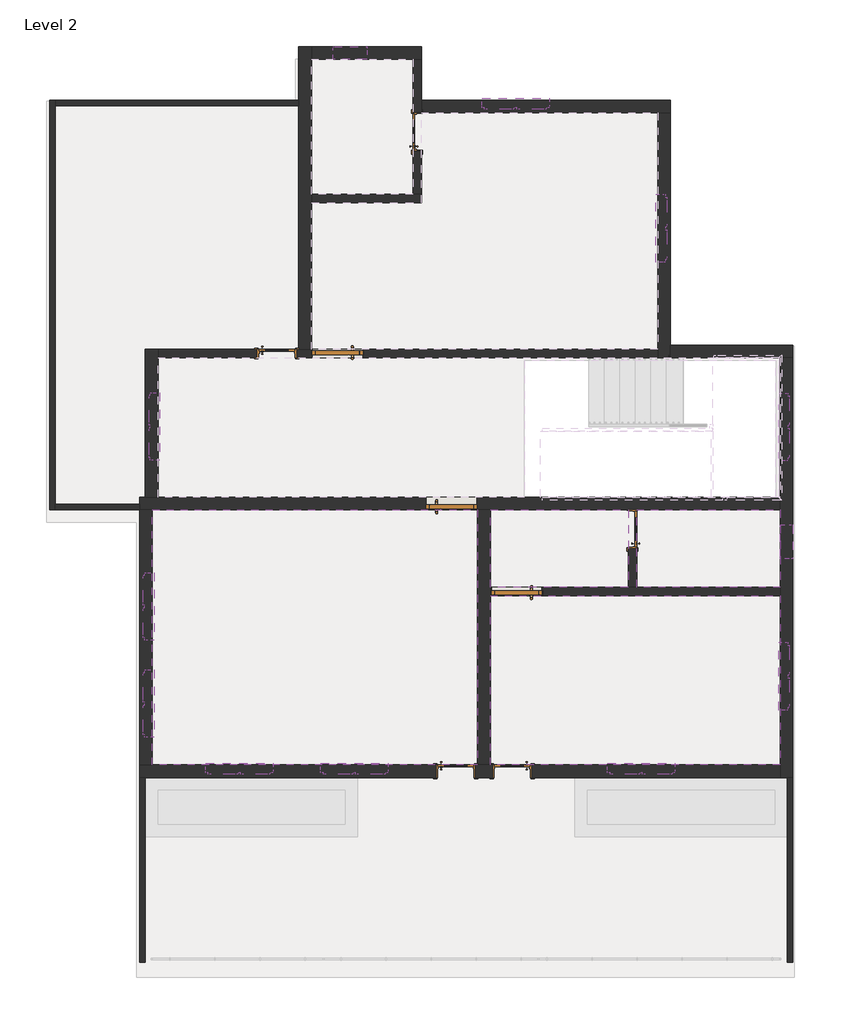
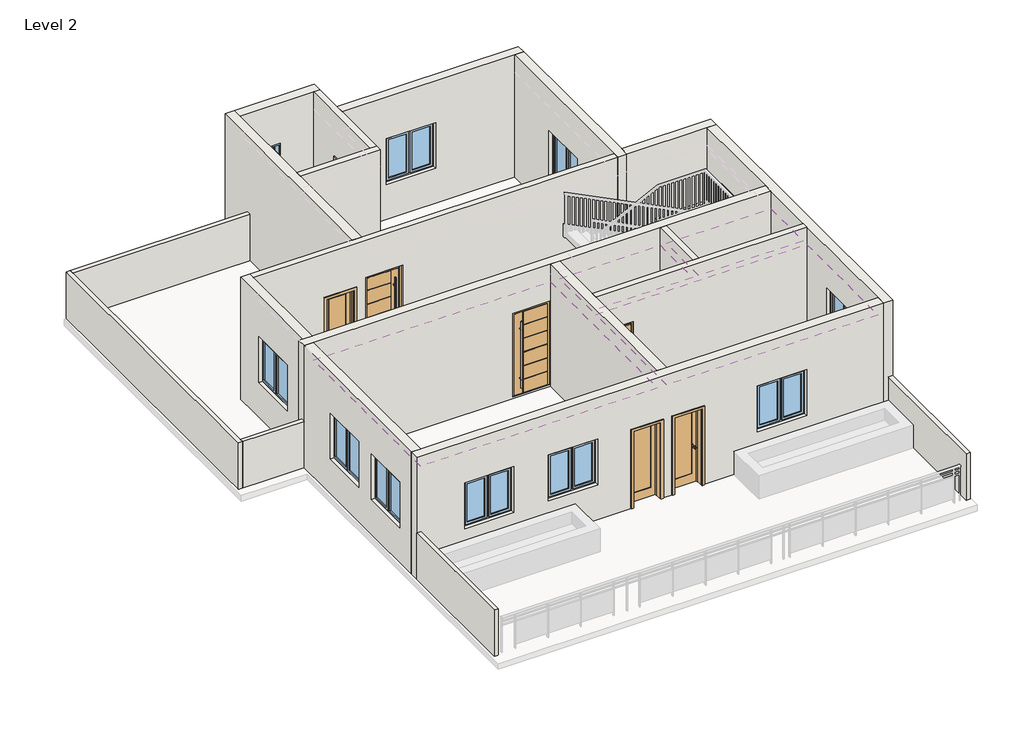
# One storey, part 1 of 3: 21 walls, 12 windows, 8 doors, 4 coverings.
"""IFC4 building model written with IfcOpenShell, lengths in millimetres."""

from ifc_helpers import new_model, si_unit, frame, origin, place, context, project, spatial, polyline, outline, extrude, faceted_brep, transform, mapped, element, save
from components import door_3_5c4206ef, door_3_79df91aa, door_3_130b8d4e, door_69f71937, door_acb0f330, door_a93bef0d, door_ae2d502c, awning_casement_double_4_37d249be, fixed_2_8c8825d0

model = new_model("IFC4")

# Units and contexts
model_context = context("Model", 3, world=origin())
ifc_project = project(units=[si_unit("LENGTHUNIT", "METRE", prefix="MILLI")], contexts=[model_context])

# Site, building, storey
site = spatial("IfcSite", under=ifc_project)
building = spatial("IfcBuilding", under=site)
storey = spatial("IfcBuildingStorey", under=building, Name="Level 2", Elevation=3200.4)

# Coverings
placement = place(None, origin())
element("IfcCovering", 1, ObjectType="2' x 4' ACT System", at=placement, inside=storey, context=model_context, shape_type="SweptSolid", body=[
    extrude(outline(polyline([(-14175.8183666, 640.5503619), (-14175.8183666, -3956.8496381), (-20043.2183666, -3956.8496381), (-20043.2183666, 640.5503619), (-14175.8183666, 640.5503619)])), frame((0.0, 0.0, 6248.4), z_axis=(0.0, 0.0, 1.0), x_axis=(1.0, 0.0, 0.0)), (0.0, 0.0, 1.0), 57.15),
])
element("IfcCovering", 2, ObjectType="2' x 4' ACT System", at=placement, inside=storey, context=model_context, shape_type="SweptSolid", body=[
    extrude(outline(polyline([(-13947.2183666, 640.5503619), (-11458.0183666, 640.5503619), (-11458.0183666, -756.4496381), (-13947.2183666, -756.4496381), (-13947.2183666, 640.5503619)])), frame((0.0, 0.0, 6248.4), z_axis=(0.0, 0.0, 1.0), x_axis=(1.0, 0.0, 0.0)), (0.0, 0.0, 1.0), 57.15),
])
element("IfcCovering", 3, ObjectType="2' x 4' ACT System", at=placement, inside=storey, context=model_context, shape_type="SweptSolid", body=[
    extrude(outline(polyline([(-8714.8183666, 640.5503619), (-8714.8183666, -756.4496381), (-11305.6183666, -756.4496381), (-11305.6183666, 640.5503619), (-8714.8183666, 640.5503619)])), frame((0.0, 0.0, 6248.4), z_axis=(0.0, 0.0, 1.0), x_axis=(1.0, 0.0, 0.0)), (0.0, 0.0, 1.0), 57.15),
])
element("IfcCovering", 4, ObjectType="2' x 4' ACT System", at=placement, inside=storey, context=model_context, shape_type="SweptSolid", body=[
    extrude(outline(polyline([(-13947.2183666, -908.8496381), (-8714.8183666, -908.8496381), (-8714.8183666, -3956.8496381), (-13947.2183666, -3956.8496381), (-13947.2183666, -908.8496381)])), frame((0.0, 0.0, 6248.4), z_axis=(0.0, 0.0, 1.0), x_axis=(1.0, 0.0, 0.0)), (0.0, 0.0, 1.0), 57.15),
])

# Doors
door_3_shape = door_3_5c4206ef(model_context)
element("IfcDoor", 5, ObjectType="3'", at=placement, inside=storey, context=model_context, shape_type="MappedRepresentation", body=[
    mapped(door_3_shape, transform((-13470.9683666, -832.6496381, 3551.4445349), x_axis=(-1.0, 0.0, 0.0), y_axis=(0.0, -1.0, 0.0), z_axis=(0.0, 0.0, 1.0))),
])
door_3_2_shape = door_3_79df91aa(model_context)
element("IfcDoor", 6, ObjectType="3'", at=placement, inside=storey, context=model_context, shape_type="MappedRepresentation", body=[
    mapped(door_3_2_shape, transform((-16703.1183666, 3459.9503619, 3551.4445349), x_axis=(-1.0, 0.0, 0.0), y_axis=(0.0, -1.0, 0.0), z_axis=(0.0, 0.0, 1.0))),
])
door_3_3_shape = door_3_130b8d4e(model_context)
element("IfcDoor", 7, ObjectType="3'", at=placement, inside=storey, context=model_context, shape_type="MappedRepresentation", body=[
    mapped(door_3_3_shape, transform((-14645.7183666, 754.8503619, 3551.4445349), x_axis=(1.0, 0.0, 0.0), y_axis=(0.0, 1.0, 0.0), z_axis=(0.0, 0.0, 1.0))),
])
door_shape = door_69f71937(model_context)
element("IfcDoor", 8, ObjectType="M_Door-Interior-Single-1_Panel-Wood : 2'2\"", at=placement, inside=storey, context=model_context, shape_type="MappedRepresentation", body=[
    mapped(door_shape, transform((-17795.3183666, 3463.1253619, 3505.2), x_axis=(1.0, 0.0, 0.0), y_axis=(0.0, 1.0, 0.0), z_axis=(0.0, 0.0, 1.0))),
])
element("IfcDoor", 9, ObjectType="M_Door-Interior-Single-1_Panel-Wood : 2'2\"", at=placement, inside=storey, context=model_context, shape_type="MappedRepresentation", body=[
    mapped(door_shape, transform((-15271.1933666, 7460.4503619, 3505.2), x_axis=(0.0, 1.0, 0.0), y_axis=(-1.0, 0.0, 0.0), z_axis=(0.0, 0.0, 1.0))),
])
door_2_shape = door_acb0f330(model_context)
element("IfcDoor", 10, ObjectType="M_Door-Interior-Single-1_Panel-Wood : 2'2\"", at=placement, inside=storey, context=model_context, shape_type="MappedRepresentation", body=[
    mapped(door_2_shape, transform((-11378.6433666, 297.6503619, 3505.2), x_axis=(0.0, 1.0, 0.0), y_axis=(-1.0, 0.0, 0.0), z_axis=(0.0, 0.0, 1.0))),
])
door_4_shape = door_a93bef0d(model_context)
element("IfcDoor", 11, ObjectType="M_Door-Interior-Single-1_Panel-Wood : 2'2\"", at=placement, inside=storey, context=model_context, shape_type="MappedRepresentation", body=[
    mapped(door_4_shape, transform((-13553.5183666, -4067.9746381, 3505.2), x_axis=(-1.0, 0.0, 0.0), y_axis=(0.0, -1.0, 0.0), z_axis=(0.0, 0.0, 1.0))),
])
door_5_shape = door_ae2d502c(model_context)
element("IfcDoor", 12, ObjectType="M_Door-Interior-Single-1_Panel-Wood : 2'2\"", at=placement, inside=storey, context=model_context, shape_type="MappedRepresentation", body=[
    mapped(door_5_shape, transform((-14569.5183666, -4067.9746381, 3505.2), x_axis=(1.0, 0.0, 0.0), y_axis=(0.0, 1.0, 0.0), z_axis=(0.0, 0.0, 1.0))),
])

# Walls
element("IfcWall", 13, ObjectType="Generic - 4\"", at=placement, inside=storey, context=model_context, shape_type="Brep", body=[
    faceted_brep([(-21897.4183666, 8031.9503619, 3505.2), (-21897.4183666, 640.5503619, 3505.2), (-21897.4183666, 640.5503619, 4724.4), (-21897.4183666, 8031.9503619, 4724.4), (-21795.8183666, 8031.9503619, 3505.2), (-21795.8183666, 8031.9503619, 4724.4), (-21795.8183666, 7930.3503619, 4724.4), (-21795.8183666, 742.1503619, 4724.4), (-21795.8183666, 640.5503619, 4724.4), (-21795.8183666, 640.5503619, 3505.2), (-21795.8183666, 742.1503619, 3505.2), (-21795.8183666, 7930.3503619, 3505.2)], [[[0, 1, 2, 3]], [[4, 5, 6, 7, 8, 9, 10, 11]], [[1, 0, 4, 11, 10, 9]], [[3, 2, 8, 7, 6, 5]], [[2, 1, 9, 8]], [[0, 3, 5, 4]]]),
])
element("IfcWall", 14, ObjectType="Generic - 4\"", at=placement, inside=storey, context=model_context, shape_type="SweptSolid", body=[
    extrude(outline(polyline([(-20271.8183666, 640.5503619), (-21795.8183666, 640.5503619), (-21795.8183666, 742.1503619), (-20271.8183666, 742.1503619), (-20271.8183666, 640.5503619)])), frame((0.0, 0.0, 3505.2), z_axis=(0.0, 0.0, 1.0), x_axis=(1.0, 0.0, 0.0)), (0.0, 0.0, 1.0), 1219.2),
])
element("IfcWall", 15, ObjectType="Generic - 4\"", at=placement, inside=storey, context=model_context, shape_type="SweptSolid", body=[
    extrude(outline(polyline([(-17401.6183666, 7930.3503619), (-21795.8183666, 7930.3503619), (-21795.8183666, 8031.9503619), (-17401.6183666, 8031.9503619), (-17401.6183666, 7930.3503619)])), frame((0.0, 0.0, 3505.2), z_axis=(0.0, 0.0, 1.0), x_axis=(1.0, 0.0, 0.0)), (0.0, 0.0, 1.0), 1219.2),
])
element("IfcWall", 16, ObjectType="Generic - 4\"", at=placement, inside=storey, context=model_context, shape_type="SweptSolid", body=[
    extrude(outline(polyline([(-20271.8183666, -7512.8496381), (-20271.8183666, -4185.4496381), (-20170.2183666, -4185.4496381), (-20170.2183666, -7512.8496381), (-20271.8183666, -7512.8496381)])), frame((0.0, 0.0, 3505.2), z_axis=(0.0, 0.0, 1.0), x_axis=(1.0, 0.0, 0.0)), (0.0, 0.0, 1.0), 1219.2),
])
element("IfcWall", 17, ObjectType="Generic - 4\"", at=placement, inside=storey, context=model_context, shape_type="SweptSolid", body=[
    extrude(outline(polyline([(-8486.2183666, -4185.4496381), (-8486.2183666, -7512.8496381), (-8587.8183666, -7512.8496381), (-8587.8183666, -4185.4496381), (-8486.2183666, -4185.4496381)])), frame((0.0, 0.0, 3505.2), z_axis=(0.0, 0.0, 1.0), x_axis=(1.0, 0.0, 0.0)), (0.0, 0.0, 1.0), 1219.2),
])
element("IfcWall", 18, ObjectType="Generic - 6\"", at=placement, inside=storey, context=model_context, shape_type="Brep", body=[
    faceted_brep([(-15344.2183666, 6330.1503619, 6705.6), (-15344.2183666, 8768.5503619, 6705.6), (-15344.2183666, 8768.5503619, 3505.2), (-15344.2183666, 7815.6503619, 3505.2), (-15344.2183666, 7815.6503619, 5530.2), (-15344.2183666, 7105.2503619, 5530.2), (-15344.2183666, 7105.2503619, 3505.2), (-15344.2183666, 6330.1503619, 3505.2), (-15191.8183666, 8768.5503619, 6705.6), (-15191.8183666, 8031.9503619, 6705.6), (-15191.8183666, 7803.3503619, 6705.6), (-15191.8183666, 6330.1503619, 6705.6), (-15191.8183666, 6330.1503619, 3505.2), (-15191.8183666, 7105.2503619, 3505.2), (-15191.8183666, 7105.2503619, 5530.2), (-15191.8183666, 7815.6503619, 5530.2), (-15191.8183666, 7815.6503619, 3505.2), (-15191.8183666, 8031.9503619, 3505.2), (-15191.8183666, 8768.5503619, 3505.2)], [[[0, 1, 2, 3, 4, 5, 6, 7]], [[8, 9, 10, 11, 12, 13, 14, 15, 16, 17, 18]], [[2, 18, 17, 16, 3]], [[12, 7, 6, 13]], [[1, 0, 11, 10, 9, 8]], [[2, 1, 8, 18]], [[0, 7, 12, 11]], [[15, 4, 3, 16]], [[4, 15, 14, 5]], [[5, 14, 13, 6]]]),
])
element("IfcWall", 19, ObjectType="Generic - 6\"", at=placement, inside=storey, context=model_context, shape_type="Brep", body=[
    faceted_brep([(-10924.6183666, 3383.7503619, 6705.6), (-19941.6183666, 3383.7503619, 6705.6), (-19941.6183666, 3383.7503619, 3505.2), (-18150.5183666, 3383.7503619, 3505.2), (-18150.5183666, 3383.7503619, 5530.2), (-17440.1183666, 3383.7503619, 5530.2), (-17440.1183666, 3383.7503619, 3505.2), (-10924.6183666, 3383.7503619, 3505.2), (-17160.3183666, 3383.7503619, 5740.9445349), (-16245.9183666, 3383.7503619, 5740.9445349), (-16245.9183666, 3383.7503619, 3551.4445349), (-17160.3183666, 3383.7503619, 3551.4445349), (-19941.6183666, 3536.1503619, 6705.6), (-17401.6183666, 3536.1503619, 6705.6), (-17173.0183666, 3536.1503619, 6705.6), (-10924.6183666, 3536.1503619, 6705.6), (-10924.6183666, 3536.1503619, 3505.2), (-17173.0183666, 3536.1503619, 3505.2), (-17401.6183666, 3536.1503619, 3505.2), (-17440.1183666, 3536.1503619, 3505.2), (-17440.1183666, 3536.1503619, 5530.2), (-18150.5183666, 3536.1503619, 5530.2), (-18150.5183666, 3536.1503619, 3505.2), (-19941.6183666, 3536.1503619, 3505.2), (-16245.9183666, 3536.1503619, 5740.9445349), (-17160.3183666, 3536.1503619, 5740.9445349), (-17160.3183666, 3536.1503619, 3551.4445349), (-16245.9183666, 3536.1503619, 3551.4445349), (-16245.9183666, 3516.1503619, 5740.9445349), (-17160.3183666, 3516.1503619, 5740.9445349), (-17160.3183666, 3439.1503619, 5740.9445349), (-16245.9183666, 3439.1503619, 5740.9445349), (-17160.3183666, 3516.1503619, 3551.4445349), (-17160.3183666, 3439.1503619, 3551.4445349), (-17175.3183666, 3516.1503619, 3551.4445349), (-17175.3183666, 3439.1503619, 3551.4445349), (-16245.9183666, 3439.1503619, 3551.4445349), (-16230.9183666, 3439.1503619, 3551.4445349), (-16230.9183666, 3516.1503619, 3551.4445349), (-16245.9183666, 3516.1503619, 3551.4445349), (-16230.9183666, 3516.1503619, 5755.9445349), (-16230.9183666, 3439.1503619, 5755.9445349), (-17175.3183666, 3439.1503619, 5755.9445349), (-17175.3183666, 3516.1503619, 5755.9445349)], [[[0, 1, 2, 3, 4, 5, 6, 7], [8, 9, 10, 11]], [[12, 13, 14, 15, 16, 17, 18, 19, 20, 21, 22, 23], [24, 25, 26, 27]], [[2, 23, 22, 3]], [[16, 7, 6, 19, 18, 17]], [[1, 0, 15, 14, 13, 12]], [[0, 7, 16, 15]], [[2, 1, 12, 23]], [[5, 20, 19, 6]], [[20, 5, 4, 21]], [[21, 4, 3, 22]], [[24, 28, 29, 25]], [[8, 30, 31, 9]], [[25, 29, 32, 26]], [[30, 8, 11, 33]], [[26, 32, 34, 35, 33, 11, 10, 36, 37, 38, 39, 27]], [[28, 24, 27, 39]], [[9, 31, 36, 10]], [[40, 41, 42, 43]], [[35, 34, 43, 42]], [[31, 30, 33, 35, 42, 41, 37, 36]], [[38, 37, 41, 40]], [[29, 28, 39, 38, 40, 43, 34, 32]]]),
])
element("IfcWall", 20, ObjectType="Generic - 6\"", at=placement, inside=storey, context=model_context, shape_type="Brep", body=[
    faceted_brep([(-17173.0183666, 6177.7503619, 3505.2), (-15191.8183666, 6177.7503619, 3505.2), (-15191.8183666, 6177.7503619, 6705.6), (-17173.0183666, 6177.7503619, 6705.6), (-17173.0183666, 6330.1503619, 3505.2), (-17173.0183666, 6330.1503619, 6705.6), (-15344.2183666, 6330.1503619, 6705.6), (-15191.8183666, 6330.1503619, 6705.6), (-15191.8183666, 6330.1503619, 3505.2), (-15344.2183666, 6330.1503619, 3505.2)], [[[0, 1, 2, 3]], [[4, 5, 6, 7, 8, 9]], [[1, 0, 4, 9, 8]], [[3, 2, 7, 6, 5]], [[0, 3, 5, 4]], [[2, 1, 8, 7]]]),
])
element("IfcWall", 21, ObjectType="Generic - 6\"", at=placement, inside=storey, context=model_context, shape_type="Brep", body=[
    faceted_brep([(-8714.8183666, -756.4496381, 3505.2), (-11305.6183666, -756.4496381, 3505.2), (-11458.0183666, -756.4496381, 3505.2), (-13947.2183666, -756.4496381, 3505.2), (-13947.2183666, -756.4496381, 6705.6), (-11458.0183666, -756.4496381, 6705.6), (-11305.6183666, -756.4496381, 6705.6), (-8714.8183666, -756.4496381, 6705.6), (-13013.7683666, -756.4496381, 5740.9445349), (-13928.1683666, -756.4496381, 5740.9445349), (-13928.1683666, -756.4496381, 3551.4445349), (-13013.7683666, -756.4496381, 3551.4445349), (-13947.2183666, -908.8496381, 3505.2), (-8714.8183666, -908.8496381, 3505.2), (-8714.8183666, -908.8496381, 6705.6), (-13947.2183666, -908.8496381, 6705.6), (-13928.1683666, -908.8496381, 5740.9445349), (-13013.7683666, -908.8496381, 5740.9445349), (-13013.7683666, -908.8496381, 3551.4445349), (-13928.1683666, -908.8496381, 3551.4445349), (-13928.1683666, -888.8496381, 5740.9445349), (-13013.7683666, -888.8496381, 5740.9445349), (-13013.7683666, -811.8496381, 5740.9445349), (-13928.1683666, -811.8496381, 5740.9445349), (-13928.1683666, -888.8496381, 3551.4445349), (-13928.1683666, -811.8496381, 3551.4445349), (-13013.7683666, -888.8496381, 3551.4445349), (-12998.7683666, -888.8496381, 3551.4445349), (-12998.7683666, -811.8496381, 3551.4445349), (-13013.7683666, -811.8496381, 3551.4445349), (-13943.1683666, -811.8496381, 3551.4445349), (-13943.1683666, -888.8496381, 3551.4445349), (-12998.7683666, -888.8496381, 5755.9445349), (-13943.1683666, -888.8496381, 5755.9445349), (-13943.1683666, -811.8496381, 5755.9445349), (-12998.7683666, -811.8496381, 5755.9445349)], [[[0, 1, 2, 3, 4, 5, 6, 7], [8, 9, 10, 11]], [[12, 13, 14, 15], [16, 17, 18, 19]], [[3, 2, 1, 0, 13, 12]], [[7, 6, 5, 4, 15, 14]], [[0, 7, 14, 13]], [[4, 3, 12, 15]], [[16, 20, 21, 17]], [[8, 22, 23, 9]], [[20, 16, 19, 24]], [[9, 23, 25, 10]], [[24, 19, 18, 26, 27, 28, 29, 11, 10, 25, 30, 31]], [[17, 21, 26, 18]], [[22, 8, 11, 29]], [[32, 33, 34, 35]], [[31, 30, 34, 33]], [[23, 22, 29, 28, 35, 34, 30, 25]], [[28, 27, 32, 35]], [[21, 20, 24, 31, 33, 32, 27, 26]]]),
])
element("IfcWall", 22, ObjectType="Generic - 6\"", at=placement, inside=storey, context=model_context, shape_type="SweptSolid", body=[
    extrude(outline(polyline([(-756.4496381, 6705.6), (640.5503619, 6705.6), (640.5503619, 5530.2), (-57.5496381, 5530.2), (-57.5496381, 3505.2), (-756.4496381, 3505.2), (-756.4496381, 6705.6)])), frame((-11458.0183666, 0.0, 0.0), z_axis=(1.0, 0.0, 0.0), x_axis=(0.0, 1.0, 0.0)), (0.0, 0.0, 1.0), 152.4),
])
element("IfcWall", 23, ObjectType="Generic - 9\"", at=placement, inside=storey, context=model_context, shape_type="Brep", body=[
    faceted_brep([(-17173.0183666, 3536.1503619, 3505.2), (-17173.0183666, 6177.7503619, 3505.2), (-17173.0183666, 6330.1503619, 3505.2), (-17173.0183666, 8768.5503619, 3505.2), (-17173.0183666, 8997.1503619, 3505.2), (-17173.0183666, 8997.1503619, 6705.6), (-17173.0183666, 8768.5503619, 6705.6), (-17173.0183666, 6330.1503619, 6705.6), (-17173.0183666, 6177.7503619, 6705.6), (-17173.0183666, 3536.1503619, 6705.6), (-17401.6183666, 3536.1503619, 3505.2), (-17401.6183666, 3536.1503619, 6705.6), (-17401.6183666, 8997.1503619, 6705.6), (-17401.6183666, 8997.1503619, 3505.2), (-17401.6183666, 8031.9503619, 3505.2), (-17401.6183666, 7930.3503619, 3505.2)], [[[0, 1, 2, 3, 4, 5, 6, 7, 8, 9]], [[10, 11, 12, 13, 14, 15]], [[4, 3, 2, 1, 0, 10, 15, 14, 13]], [[9, 8, 7, 6, 5, 12, 11]], [[5, 4, 13, 12]], [[0, 9, 11, 10]]]),
])
element("IfcWall", 24, ObjectType="Generic - 9\"", at=placement, inside=storey, context=model_context, shape_type="Brep", body=[
    faceted_brep([(-17173.0183666, 8768.5503619, 3505.2), (-15344.2183666, 8768.5503619, 3505.2), (-15191.8183666, 8768.5503619, 3505.2), (-15191.8183666, 8768.5503619, 6705.6), (-15344.2183666, 8768.5503619, 6705.6), (-17173.0183666, 8768.5503619, 6705.6), (-16169.7183666, 8768.5503619, 5638.8), (-16169.7183666, 8768.5503619, 5334.0), (-16779.3183666, 8768.5503619, 5334.0), (-16779.3183666, 8768.5503619, 5638.8), (-17173.0183666, 8997.1503619, 3505.2), (-17173.0183666, 8997.1503619, 6705.6), (-15191.8183666, 8997.1503619, 6705.6), (-15191.8183666, 8997.1503619, 3505.2), (-16169.7183666, 8997.1503619, 5638.8), (-16779.3183666, 8997.1503619, 5638.8), (-16779.3183666, 8997.1503619, 5334.0), (-16169.7183666, 8997.1503619, 5334.0)], [[[0, 1, 2, 3, 4, 5], [6, 7, 8, 9]], [[10, 11, 12, 13], [14, 15, 16, 17]], [[2, 1, 0, 10, 13]], [[5, 4, 3, 12, 11]], [[0, 5, 11, 10]], [[3, 2, 13, 12]], [[7, 6, 14, 17]], [[8, 7, 17, 16]], [[9, 8, 16, 15]], [[6, 9, 15, 14]]]),
])
element("IfcWall", 25, ObjectType="Generic - 9\"", at=placement, inside=storey, context=model_context, shape_type="Brep", body=[
    faceted_brep([(-15191.8183666, 7803.3503619, 3505.2), (-10924.6183666, 7803.3503619, 3505.2), (-10696.0183666, 7803.3503619, 3505.2), (-10696.0183666, 7803.3503619, 6705.6), (-10924.6183666, 7803.3503619, 6705.6), (-15191.8183666, 7803.3503619, 6705.6), (-14099.6183666, 7803.3503619, 4419.6), (-14099.6183666, 7803.3503619, 5619.6), (-12880.4183666, 7803.3503619, 5619.6), (-12880.4183666, 7803.3503619, 4419.6), (-15191.8183666, 8031.9503619, 3505.2), (-15191.8183666, 8031.9503619, 6705.6), (-10696.0183666, 8031.9503619, 6705.6), (-10696.0183666, 8031.9503619, 3505.2), (-14099.6183666, 8031.9503619, 4419.6), (-12880.4183666, 8031.9503619, 4419.6), (-12880.4183666, 8031.9503619, 5619.6), (-14099.6183666, 8031.9503619, 5619.6)], [[[0, 1, 2, 3, 4, 5], [6, 7, 8, 9]], [[10, 11, 12, 13], [14, 15, 16, 17]], [[2, 1, 0, 10, 13]], [[5, 4, 3, 12, 11]], [[0, 5, 11, 10]], [[3, 2, 13, 12]], [[7, 6, 14, 17]], [[8, 7, 17, 16]], [[9, 8, 16, 15]], [[6, 9, 15, 14]]]),
])
element("IfcWall", 26, ObjectType="Generic - 9\"", at=placement, inside=storey, context=model_context, shape_type="Brep", body=[
    faceted_brep([(-10924.6183666, 7803.3503619, 3505.2), (-10924.6183666, 3536.1503619, 3505.2), (-10924.6183666, 3383.7503619, 3505.2), (-10924.6183666, 3383.7503619, 6705.6), (-10924.6183666, 3536.1503619, 6705.6), (-10924.6183666, 7803.3503619, 6705.6), (-10924.6183666, 5110.9503619, 4419.6), (-10924.6183666, 6330.1503619, 4419.6), (-10924.6183666, 6330.1503619, 5619.6), (-10924.6183666, 5110.9503619, 5619.6), (-10696.0183666, 7803.3503619, 3505.2), (-10696.0183666, 7803.3503619, 6705.6), (-10696.0183666, 3612.3503619, 6705.6), (-10696.0183666, 3383.7503619, 6705.6), (-10696.0183666, 3383.7503619, 3505.2), (-10696.0183666, 3612.3503619, 3505.2), (-10696.0183666, 5110.9503619, 4419.6), (-10696.0183666, 5110.9503619, 5619.6), (-10696.0183666, 6330.1503619, 5619.6), (-10696.0183666, 6330.1503619, 4419.6)], [[[0, 1, 2, 3, 4, 5], [6, 7, 8, 9]], [[10, 11, 12, 13, 14, 15], [16, 17, 18, 19]], [[2, 1, 0, 10, 15, 14]], [[5, 4, 3, 13, 12, 11]], [[0, 5, 11, 10]], [[3, 2, 14, 13]], [[17, 16, 6, 9]], [[18, 17, 9, 8]], [[19, 18, 8, 7]], [[16, 19, 7, 6]]]),
])
element("IfcWall", 27, ObjectType="Generic - 9\"", at=placement, inside=storey, context=model_context, shape_type="Brep", body=[
    faceted_brep([(-10696.0183666, 3383.7503619, 3505.2), (-8714.8183666, 3383.7503619, 3505.2), (-8486.2183666, 3383.7503619, 3505.2), (-8486.2183666, 3383.7503619, 6705.6), (-8714.8183666, 3383.7503619, 6705.6), (-10696.0183666, 3383.7503619, 6705.6), (-10696.0183666, 3612.3503619, 3505.2), (-10696.0183666, 3612.3503619, 6705.6), (-8486.2183666, 3612.3503619, 6705.6), (-8486.2183666, 3612.3503619, 3505.2)], [[[0, 1, 2, 3, 4, 5]], [[6, 7, 8, 9]], [[2, 1, 0, 6, 9]], [[5, 4, 3, 8, 7]], [[0, 5, 7, 6]], [[3, 2, 9, 8]]]),
])
element("IfcWall", 28, ObjectType="Generic - 9\"", at=placement, inside=storey, context=model_context, shape_type="Brep", body=[
    faceted_brep([(-8714.8183666, 3383.7503619, 3505.2), (-8714.8183666, 869.1503619, 3505.2), (-8714.8183666, 640.5503619, 3505.2), (-8714.8183666, -756.4496381, 3505.2), (-8714.8183666, -908.8496381, 3505.2), (-8714.8183666, -3956.8496381, 3505.2), (-8714.8183666, -4185.4496381, 3505.2), (-8714.8183666, -4185.4496381, 6705.6), (-8714.8183666, -3956.8496381, 6705.6), (-8714.8183666, -908.8496381, 6705.6), (-8714.8183666, -756.4496381, 6705.6), (-8714.8183666, 640.5503619, 6705.6), (-8714.8183666, 869.1503619, 6705.6), (-8714.8183666, 3383.7503619, 6705.6), (-8714.8183666, -2966.2496381, 4419.6), (-8714.8183666, -1747.0496381, 4419.6), (-8714.8183666, -1747.0496381, 5619.6), (-8714.8183666, -2966.2496381, 5619.6), (-8714.8183666, 1529.5503619, 4419.6), (-8714.8183666, 2748.7503619, 4419.6), (-8714.8183666, 2748.7503619, 5619.6), (-8714.8183666, 1529.5503619, 5619.6), (-8714.8183666, -235.7496381, 5638.8), (-8714.8183666, -235.7496381, 5334.0), (-8714.8183666, 373.8503619, 5334.0), (-8714.8183666, 373.8503619, 5638.8), (-8486.2183666, 3383.7503619, 3505.2), (-8486.2183666, 3383.7503619, 6705.6), (-8486.2183666, -4185.4496381, 6705.6), (-8486.2183666, -4185.4496381, 4724.4), (-8486.2183666, -4185.4496381, 3505.2), (-8486.2183666, -2966.2496381, 4419.6), (-8486.2183666, -2966.2496381, 5619.6), (-8486.2183666, -1747.0496381, 5619.6), (-8486.2183666, -1747.0496381, 4419.6), (-8486.2183666, 1529.5503619, 4419.6), (-8486.2183666, 1529.5503619, 5619.6), (-8486.2183666, 2748.7503619, 5619.6), (-8486.2183666, 2748.7503619, 4419.6), (-8486.2183666, -235.7496381, 5638.8), (-8486.2183666, 373.8503619, 5638.8), (-8486.2183666, 373.8503619, 5334.0), (-8486.2183666, -235.7496381, 5334.0), (-8587.8183666, -4185.4496381, 3505.2)], [[[0, 1, 2, 3, 4, 5, 6, 7, 8, 9, 10, 11, 12, 13], [14, 15, 16, 17], [18, 19, 20, 21], [22, 23, 24, 25]], [[26, 27, 28, 29, 30], [31, 32, 33, 34], [35, 36, 37, 38], [39, 40, 41, 42]], [[6, 5, 4, 3, 2, 1, 0, 26, 30, 43]], [[13, 12, 11, 10, 9, 8, 7, 28, 27]], [[0, 13, 27, 26]], [[6, 43, 30, 29, 28, 7]], [[32, 31, 14, 17]], [[33, 32, 17, 16]], [[34, 33, 16, 15]], [[31, 34, 15, 14]], [[36, 35, 18, 21]], [[37, 36, 21, 20]], [[38, 37, 20, 19]], [[35, 38, 19, 18]], [[23, 22, 39, 42]], [[24, 23, 42, 41]], [[25, 24, 41, 40]], [[22, 25, 40, 39]]]),
])
element("IfcWall", 29, ObjectType="Generic - 9\"", at=placement, inside=storey, context=model_context, shape_type="Brep", body=[
    faceted_brep([(-20272.0228179, -3956.8496381, 3505.2), (-20272.0228179, -3956.8496381, 6705.6), (-20271.8183666, -3956.8496381, 6705.6), (-20043.2183666, -3956.8496381, 6705.6), (-14175.8183666, -3956.8496381, 6705.6), (-13947.2183666, -3956.8496381, 6705.6), (-8714.8183666, -3956.8496381, 6705.6), (-8714.8183666, -3956.8496381, 3505.2), (-13198.3183666, -3956.8496381, 3505.2), (-13198.3183666, -3956.8496381, 5530.2), (-13908.7183666, -3956.8496381, 5530.2), (-13908.7183666, -3956.8496381, 3505.2), (-13947.2183666, -3956.8496381, 3505.2), (-14175.8183666, -3956.8496381, 3505.2), (-14214.3183666, -3956.8496381, 3505.2), (-14214.3183666, -3956.8496381, 5530.2), (-14924.7183666, -3956.8496381, 5530.2), (-14924.7183666, -3956.8496381, 3505.2), (-20043.2183666, -3956.8496381, 3505.2), (-20271.8183666, -3956.8496381, 3505.2), (-19084.3683666, -3956.8496381, 4419.6), (-17865.1683666, -3956.8496381, 4419.6), (-17865.1683666, -3956.8496381, 5619.6), (-19084.3683666, -3956.8496381, 5619.6), (-17007.9183666, -3956.8496381, 4419.6), (-15788.7183666, -3956.8496381, 4419.6), (-15788.7183666, -3956.8496381, 5619.6), (-17007.9183666, -3956.8496381, 5619.6), (-11832.6683666, -3956.8496381, 4419.6), (-10613.4683666, -3956.8496381, 4419.6), (-10613.4683666, -3956.8496381, 5619.6), (-11832.6683666, -3956.8496381, 5619.6), (-20272.0228179, -4185.4496381, 6705.6), (-20272.0228179, -4185.4496381, 3505.2), (-20271.8183666, -4185.4496381, 3505.2), (-20170.2183666, -4185.4496381, 3505.2), (-14924.7183666, -4185.4496381, 3505.2), (-14924.7183666, -4185.4496381, 5530.2), (-14214.3183666, -4185.4496381, 5530.2), (-14214.3183666, -4185.4496381, 3505.2), (-13908.7183666, -4185.4496381, 3505.2), (-13908.7183666, -4185.4496381, 5530.2), (-13198.3183666, -4185.4496381, 5530.2), (-13198.3183666, -4185.4496381, 3505.2), (-8714.8183666, -4185.4496381, 3505.2), (-8714.8183666, -4185.4496381, 6705.6), (-19084.3683666, -4185.4496381, 4419.6), (-19084.3683666, -4185.4496381, 5619.6), (-17865.1683666, -4185.4496381, 5619.6), (-17865.1683666, -4185.4496381, 4419.6), (-17007.9183666, -4185.4496381, 4419.6), (-17007.9183666, -4185.4496381, 5619.6), (-15788.7183666, -4185.4496381, 5619.6), (-15788.7183666, -4185.4496381, 4419.6), (-11832.6683666, -4185.4496381, 4419.6), (-11832.6683666, -4185.4496381, 5619.6), (-10613.4683666, -4185.4496381, 5619.6), (-10613.4683666, -4185.4496381, 4419.6)], [[[0, 1, 2, 3, 4, 5, 6, 7, 8, 9, 10, 11, 12, 13, 14, 15, 16, 17, 18, 19], [20, 21, 22, 23], [24, 25, 26, 27], [28, 29, 30, 31]], [[32, 33, 34, 35, 36, 37, 38, 39, 40, 41, 42, 43, 44, 45], [46, 47, 48, 49], [50, 51, 52, 53], [54, 55, 56, 57]], [[33, 0, 19, 18, 17, 36, 35, 34]], [[7, 44, 43, 8]], [[39, 14, 13, 12, 11, 40]], [[1, 0, 33, 32]], [[6, 5, 4, 3, 2, 1, 32, 45]], [[6, 45, 44, 7]], [[47, 46, 20, 23]], [[48, 47, 23, 22]], [[49, 48, 22, 21]], [[46, 49, 21, 20]], [[51, 50, 24, 27]], [[52, 51, 27, 26]], [[53, 52, 26, 25]], [[50, 53, 25, 24]], [[55, 54, 28, 31]], [[56, 55, 31, 30]], [[57, 56, 30, 29]], [[54, 57, 29, 28]], [[15, 14, 39, 38]], [[16, 15, 38, 37]], [[17, 16, 37, 36]], [[10, 41, 40, 11]], [[41, 10, 9, 42]], [[42, 9, 8, 43]]]),
])
element("IfcWall", 30, ObjectType="Generic - 9\"", at=placement, inside=storey, context=model_context, shape_type="SweptSolid", body=[
    extrude(outline(polyline([(-3956.8496381, 3505.2), (-3956.8496381, 6705.6), (640.5503619, 6705.6), (640.5503619, 3505.2), (-3956.8496381, 3505.2)]), holes=[polyline([(-489.7496381, 4419.6), (-489.7496381, 5619.6), (-1708.9496381, 5619.6), (-1708.9496381, 4419.6), (-489.7496381, 4419.6)]), polyline([(-2242.3496381, 4419.6), (-2242.3496381, 5619.6), (-3461.5496381, 5619.6), (-3461.5496381, 4419.6), (-2242.3496381, 4419.6)])]), frame((-20271.8183666, 0.0, 0.0), z_axis=(1.0, 0.0, 0.0), x_axis=(0.0, 1.0, 0.0)), (0.0, 0.0, 1.0), 228.6),
])
element("IfcWall", 31, ObjectType="Generic - 9\"", at=placement, inside=storey, context=model_context, shape_type="Brep", body=[
    faceted_brep([(-8714.8183666, 640.5503619, 6705.6), (-11305.6183666, 640.5503619, 6705.6), (-11458.0183666, 640.5503619, 6705.6), (-13947.2183666, 640.5503619, 6705.6), (-14175.8183666, 640.5503619, 6705.6), (-20043.2183666, 640.5503619, 6705.6), (-20271.8183666, 640.5503619, 6705.6), (-20271.8183666, 640.5503619, 4724.4), (-20271.8183666, 640.5503619, 3505.2), (-20043.2183666, 640.5503619, 3505.2), (-14175.8183666, 640.5503619, 3505.2), (-13947.2183666, 640.5503619, 3505.2), (-11458.0183666, 640.5503619, 3505.2), (-11458.0183666, 640.5503619, 5530.2), (-11305.6183666, 640.5503619, 5530.2), (-11305.6183666, 640.5503619, 3505.2), (-8714.8183666, 640.5503619, 3505.2), (-15102.9183666, 640.5503619, 5740.9445349), (-14188.5183666, 640.5503619, 5740.9445349), (-14188.5183666, 640.5503619, 3551.4445349), (-15102.9183666, 640.5503619, 3551.4445349), (-8714.8183666, 869.1503619, 3505.2), (-19941.6183666, 869.1503619, 3505.2), (-20170.2183666, 869.1503619, 3505.2), (-20271.8183666, 869.1503619, 3505.2), (-20271.8183666, 869.1503619, 6705.6), (-20170.2183666, 869.1503619, 6705.6), (-19941.6183666, 869.1503619, 6705.6), (-8714.8183666, 869.1503619, 6705.6), (-14188.5183666, 869.1503619, 5740.9445349), (-15102.9183666, 869.1503619, 5740.9445349), (-15102.9183666, 869.1503619, 3551.4445349), (-14188.5183666, 869.1503619, 3551.4445349), (-11305.6183666, 652.8503619, 3505.2), (-11458.0183666, 652.8503619, 3505.2), (-20271.8183666, 742.1503619, 3505.2), (-11305.6183666, 652.8503619, 5530.2), (-11458.0183666, 652.8503619, 5530.2), (-15102.9183666, 660.5503619, 5740.9445349), (-14188.5183666, 660.5503619, 5740.9445349), (-14188.5183666, 737.5503619, 5740.9445349), (-15102.9183666, 737.5503619, 5740.9445349), (-14188.5183666, 660.5503619, 3551.4445349), (-14188.5183666, 737.5503619, 3551.4445349), (-14173.5183666, 660.5503619, 3551.4445349), (-14173.5183666, 737.5503619, 3551.4445349), (-15102.9183666, 737.5503619, 3551.4445349), (-15117.9183666, 737.5503619, 3551.4445349), (-15117.9183666, 660.5503619, 3551.4445349), (-15102.9183666, 660.5503619, 3551.4445349), (-15117.9183666, 660.5503619, 5755.9445349), (-15117.9183666, 737.5503619, 5755.9445349), (-14173.5183666, 737.5503619, 5755.9445349), (-14173.5183666, 660.5503619, 5755.9445349)], [[[0, 1, 2, 3, 4, 5, 6, 7, 8, 9, 10, 11, 12, 13, 14, 15, 16], [17, 18, 19, 20]], [[21, 22, 23, 24, 25, 26, 27, 28], [29, 30, 31, 32]], [[24, 23, 22, 21, 16, 15, 33, 34, 12, 11, 10, 9, 8, 35]], [[6, 5, 4, 3, 2, 1, 0, 28, 27, 26, 25]], [[24, 35, 8, 7, 6, 25]], [[0, 16, 21, 28]], [[36, 33, 15, 14]], [[34, 37, 13, 12]], [[37, 36, 14, 13]], [[17, 38, 39, 18]], [[29, 40, 41, 30]], [[18, 39, 42, 19]], [[40, 29, 32, 43]], [[19, 42, 44, 45, 43, 32, 31, 46, 47, 48, 49, 20]], [[38, 17, 20, 49]], [[30, 41, 46, 31]], [[50, 51, 52, 53]], [[45, 44, 53, 52]], [[41, 40, 43, 45, 52, 51, 47, 46]], [[48, 47, 51, 50]], [[39, 38, 49, 48, 50, 53, 44, 42]], [[33, 36, 37, 34]]]),
])
element("IfcWall", 32, ObjectType="Generic - 9\"", at=placement, inside=storey, context=model_context, shape_type="Brep", body=[
    faceted_brep([(-19941.6183666, 869.1503619, 6705.6), (-19941.6183666, 869.1503619, 3505.2), (-19941.6183666, 3383.7503619, 3505.2), (-19941.6183666, 3536.1503619, 3505.2), (-19941.6183666, 3536.1503619, 6705.6), (-19941.6183666, 3383.7503619, 6705.6), (-19941.6183666, 2755.1003619, 4419.6), (-19941.6183666, 1535.9003619, 4419.6), (-19941.6183666, 1535.9003619, 5619.6), (-19941.6183666, 2755.1003619, 5619.6), (-20170.2183666, 869.1503619, 3505.2), (-20170.2183666, 869.1503619, 6705.6), (-20170.2183666, 3536.1503619, 6705.6), (-20170.2183666, 3536.1503619, 3505.2), (-20170.2183666, 2755.1003619, 4419.6), (-20170.2183666, 2755.1003619, 5619.6), (-20170.2183666, 1535.9003619, 5619.6), (-20170.2183666, 1535.9003619, 4419.6)], [[[0, 1, 2, 3, 4, 5], [6, 7, 8, 9]], [[10, 11, 12, 13], [14, 15, 16, 17]], [[3, 2, 1, 10, 13]], [[0, 5, 4, 12, 11]], [[0, 11, 10, 1]], [[4, 3, 13, 12]], [[15, 14, 6, 9]], [[16, 15, 9, 8]], [[17, 16, 8, 7]], [[14, 17, 7, 6]]]),
])
element("IfcWall", 33, ObjectType="Generic - 9\"", at=placement, inside=storey, context=model_context, shape_type="Brep", body=[
    faceted_brep([(-13947.2183666, -3956.8496381, 3505.2), (-13947.2183666, -908.8496381, 3505.2), (-13947.2183666, -756.4496381, 3505.2), (-13947.2183666, 640.5503619, 3505.2), (-13947.2183666, 640.5503619, 6705.6), (-13947.2183666, -756.4496381, 6705.6), (-13947.2183666, -908.8496381, 6705.6), (-13947.2183666, -3956.8496381, 6705.6), (-14175.8183666, -3956.8496381, 3505.2), (-14175.8183666, -3956.8496381, 6705.6), (-14175.8183666, 640.5503619, 6705.6), (-14175.8183666, 640.5503619, 3505.2)], [[[0, 1, 2, 3, 4, 5, 6, 7]], [[8, 9, 10, 11]], [[3, 2, 1, 0, 8, 11]], [[7, 6, 5, 4, 10, 9]], [[0, 7, 9, 8]], [[4, 3, 11, 10]]]),
])

# Windows
awning_casement_double_4_shape = awning_casement_double_4_37d249be(model_context)
element("IfcWindow", 34, ObjectType="Awning Casement double : 4'", at=placement, inside=storey, context=model_context, shape_type="MappedRepresentation", body=[
    mapped(awning_casement_double_4_shape, transform((-13490.0183666, 7917.6503619, 3619.6), x_axis=(1.0, 0.0, 0.0), y_axis=(0.0, 1.0, 0.0), z_axis=(0.0, 0.0, 1.0))),
])
element("IfcWindow", 35, ObjectType="Awning Casement double : 4'", at=placement, inside=storey, context=model_context, shape_type="MappedRepresentation", body=[
    mapped(awning_casement_double_4_shape, transform((-10810.3183666, 5720.5503619, 3619.6), x_axis=(0.0, 1.0, 0.0), y_axis=(-1.0, 0.0, 0.0), z_axis=(0.0, 0.0, 1.0))),
])
element("IfcWindow", 36, ObjectType="Awning Casement double : 4'", at=placement, inside=storey, context=model_context, shape_type="MappedRepresentation", body=[
    mapped(awning_casement_double_4_shape, transform((-20055.9183666, 2145.5003619, 3619.6), x_axis=(0.0, -1.0, 0.0), y_axis=(1.0, 0.0, 0.0), z_axis=(0.0, 0.0, 1.0))),
])
element("IfcWindow", 37, ObjectType="Awning Casement double : 4'", at=placement, inside=storey, context=model_context, shape_type="MappedRepresentation", body=[
    mapped(awning_casement_double_4_shape, transform((-20157.5183666, -1099.3496381, 3619.6), x_axis=(0.0, -1.0, 0.0), y_axis=(1.0, 0.0, 0.0), z_axis=(0.0, 0.0, 1.0))),
])
element("IfcWindow", 38, ObjectType="Awning Casement double : 4'", at=placement, inside=storey, context=model_context, shape_type="MappedRepresentation", body=[
    mapped(awning_casement_double_4_shape, transform((-20157.5183666, -2851.9496381, 3619.6), x_axis=(0.0, -1.0, 0.0), y_axis=(1.0, 0.0, 0.0), z_axis=(0.0, 0.0, 1.0))),
])
element("IfcWindow", 39, ObjectType="Awning Casement double : 4'", at=placement, inside=storey, context=model_context, shape_type="MappedRepresentation", body=[
    mapped(awning_casement_double_4_shape, transform((-18474.7683666, -4071.1496381, 3619.6), x_axis=(1.0, 0.0, 0.0), y_axis=(0.0, 1.0, 0.0), z_axis=(0.0, 0.0, 1.0))),
])
element("IfcWindow", 40, ObjectType="Awning Casement double : 4'", at=placement, inside=storey, context=model_context, shape_type="MappedRepresentation", body=[
    mapped(awning_casement_double_4_shape, transform((-16398.3183666, -4071.1496381, 3619.6), x_axis=(1.0, 0.0, 0.0), y_axis=(0.0, 1.0, 0.0), z_axis=(0.0, 0.0, 1.0))),
])
element("IfcWindow", 41, ObjectType="Awning Casement double : 4'", at=placement, inside=storey, context=model_context, shape_type="MappedRepresentation", body=[
    mapped(awning_casement_double_4_shape, transform((-11223.0683666, -4071.1496381, 3619.6), x_axis=(1.0, 0.0, 0.0), y_axis=(0.0, 1.0, 0.0), z_axis=(0.0, 0.0, 1.0))),
])
element("IfcWindow", 42, ObjectType="Awning Casement double : 4'", at=placement, inside=storey, context=model_context, shape_type="MappedRepresentation", body=[
    mapped(awning_casement_double_4_shape, transform((-8600.5183666, -2356.6496381, 3619.6), x_axis=(0.0, 1.0, 0.0), y_axis=(-1.0, 0.0, 0.0), z_axis=(0.0, 0.0, 1.0))),
])
element("IfcWindow", 43, ObjectType="Awning Casement double : 4'", at=placement, inside=storey, context=model_context, shape_type="MappedRepresentation", body=[
    mapped(awning_casement_double_4_shape, transform((-8600.5183666, 2139.1503619, 3619.6), x_axis=(0.0, 1.0, 0.0), y_axis=(-1.0, 0.0, 0.0), z_axis=(0.0, 0.0, 1.0))),
])
fixed_2_shape = fixed_2_8c8825d0(model_context)
element("IfcWindow", 44, ObjectType="Fixed : 2'", at=placement, inside=storey, context=model_context, shape_type="MappedRepresentation", body=[
    mapped(fixed_2_shape, transform((-16436.4183666, 8882.8503619, 4419.6), x_axis=(1.0, 0.0, 0.0), y_axis=(0.0, 1.0, 0.0), z_axis=(0.0, 0.0, 1.0))),
])
element("IfcWindow", 45, ObjectType="Fixed : 2'", at=placement, inside=storey, context=model_context, shape_type="MappedRepresentation", body=[
    mapped(fixed_2_shape, transform((-8600.5183666, 30.9503619, 4419.6), x_axis=(0.0, -1.0, 0.0), y_axis=(1.0, 0.0, 0.0), z_axis=(0.0, 0.0, 1.0))),
])

save(model, "model.ifc")

# Revit data of these elements
# Type "2' x 4' ACT System"
#   Assembly Code = "C3030210"
#   built-in parameter 1002203 = 1 (stored number, unit not read)
#   built-in parameter 1002202 = 1 (stored number, unit not read)
#   Layers, outside or top first: 0' - 1 5/8" "Default" (function 1); 0' - 0 5/8" "Acoustic Ceiling Tile 24 x 48" (function 5)
# Type "3'"
#   Type Mark = "15"
#   Water resistance = "up to Class E900, EN 12208:2001"
#   Uniclass2015Version = "v1.21"
#   Uniclass2015Reference = "Ss_25_30_20_30"
#   Uniclass2015Description = "Frame and door leaf system"
#   URL = "www.aluprof.com"
#   Type IFC Predefined Type = "USERDEFINED"
#   Right-hand / Left-hand door [instance default] = ""
#   Resistance to wind load = "up to Class C5/B5, EN 12210:2001"
#   Insert type = "ST"
#   Hardware [instance default] = ""
#   Product page = "https://aluprof.com/en/architects/offer/window-and-door-systems/panel-doors#visualisation"
#   Operation = "SinglePanelOutwardOpening"
#   Opening type = "Outward"
#   NBSReference = "25-50-20/125"
#   NBSDescription = "Frame and door leaf system"
#   Important = "The actual acceptable construction dimensions are dependent on the selection of profiles and hardware, glazing type, construction weight and the construction’s operating conditions. These should be determined by a suitably qualified person, and using ALUPROF’s calculation software"
#   IfcExportType = "USERDEFINED"
#   IfcExportAs = "IfcDoorType"
#   Handle type [instance default] = ""
#   Manufacturer = "ALUPROF SA"
#   Export Type to IFC As = "IfcDoorType"
#   Door sill type [instance default] = ""
#   Description = "External single-leaf panel door outward opening"
#   Model = "MB-86 ST Panel Door AD07"
#   Content of the recyclate in the material = "69.2%"
#   COBie.Type.WarrantyDurationParts = ""
#   COBie.Type.Name = ""
#   COBie.Type.Manufacturer = "ALUPROF SA"
#   COBie.Space.Name = ""
#   COBie.Floor.Name = ""
#   COBie.Facility.Name = ""
#   COBie.CreatedOn = ""
#   COBie.Component.WarrantyStartDate = ""
#   COBie.Component.Name = "MB-86 ST Panel Door AD07"
#   Burglar resistance = "RC2"
#   Air permeability = "up to Class 4, EN 12207:2001"
#   Width of the active leaf = 2' - 8.17717"
#   Placement in wall = 0' - 0.7874"
#   Thickness = 0' - 3.0315"
#   Height of the opening sash = 6' - 11.64173"
#   Handle Offset = 3' - 5.33858"
#   Rough Height = 7' - 4.61024"
#   Rough Width = 3' - 1.1811"
#   Height = 7' - 2.20079"
#   Width = 3' - 0"
#   Construction depth = 0' - 3.0315"
#   Clear opening width = 2' - 3.94882"
#   Clear opening height = 6' - 10.67717"
#   Height of the array = 1' - 1.44816"
#   Schedule No. [instance default] = 1
#   Handrail [instance default] = yes
#   IsExternal = yes
#   Handle [instance default] = no
#   Door closer [instance default] = no
#   Function = 1
#   COBie.Type = yes
#   COBie = yes
#   Access control [instance default] = no
#   Panel = element 387710
#   Wall Closure = (empty or 0)
# Type "M_Door-Interior-Single-1_Panel-Wood : 2'2\""
#   Type Mark = "17"
#   Assembly Code = "C1020300"
#   Analytic Construction = "Wooden"
#   Top Rail = 0' - 4.72441"
#   Thickness = 0' - 1.37795"
#   Thermal Resistance (R) = 2.5876 (h·ft²·°F)/BTU
#   Swing Angle [instance default] = 90.00°
#   Stiles = 0' - 4.72441"
#   Rough Width = 2' - 3.9685"
#   Rough Height = 6' - 7.72441"
#   Height = 6' - 6.74016"
#   Width = 2' - 2"
#   Heat Transfer Coefficient (U) = 0.3865 BTU/(h·ft²·°F)
#   Bottom Rail = 0' - 9.05512"
#   Trim Material = Cherry
#   Panel Material = Cherry
#   Frame Material = Cherry
#   Door Handle Material = Aluminum
#   Visual Light Transmittance = 0
#   Solar Heat Gain Coefficient = 0
#   Wall Closure = (empty or 0)
#   Function = (empty or 0)
# Type "Generic - 4\""
#   Assembly Code = "B2010"
#   Layers, outside or top first: 0' - 4" no material (function 1)
# Type "Generic - 6\""
#   Assembly Code = "B2010"
#   Layers, outside or top first: 0' - 6" no material (function 1)
# Type "Generic - 9\""
#   Assembly Code = "B2010"
#   Layers, outside or top first: 0' - 9" no material (function 1)
# Type "Awning Casement double : 4'"
#   Type Mark = "21"
#   Operation = "DoublePanelVertical"
#   Keynote = "L10/210"
#   Height = 3' - 11.24409"
#   Default Sill Height = 2' - 7.49606"
#   Width = 4' - 0"
#   Wall Closure = (empty or 0)
# Type "Fixed : 2'"
#   Type Mark = "22"
#   Construction Type Id = "GSP4R"
#   Assembly Code = "B2020100"
#   Analytic Construction = "1/8 in Pilkington single glazing"
#   Visual Light Transmittance = 0.9
#   Solar Heat Gain Coefficient = 0.78
#   Heat Transfer Coefficient (U) = 0.6496 BTU/(h·ft²·°F)
#   Height = 1' - 0"
#   Default Sill Height = 3' - 0"
#   Width = 2' - 0"
#   Window Inset = 0' - 0 3/4"
#   Define Thermal Properties by = 1
#   Glass Pane Material = Glass
#   Sash Material = Sash
#   Wall Closure = (empty or 0)
# Elements 1, 2, 3, 4 (IfcCovering, "2' x 4' ACT System")
#   Height Offset From Level = 10' - 0"
#   Phase Created = New Construction
#   Materials on its faces: "Acoustic Ceiling Tile 24 x 48", "Default"
# Elements 5, 6, 7 (IfcDoor, "3'")
#   Right-hand / Left-hand door = ""
#   Hardware = ""
#   Handle type = ""
#   Door sill type = ""
#   Schedule No. = 1
#   Handrail = yes
#   Handle = no
#   Door closer = no
#   Access control = no
#   Phase Created = New Construction
# Elements 8, 9, 10, 11, 12 (IfcDoor, "M_Door-Interior-Single-1_Panel-Wood : 2'2\"")
#   Swing Angle = 90.00°
#   Phase Created = New Construction
#   Materials on its faces: "Cherry", "Aluminum"
# Element 13 (IfcWall, "Generic - 4\"")
#   built-in parameter 1001111 = 1' - 0"
#   Top Offset = -5' - 6"
#   Base Offset = 1' - 0"
#   wall height = 4' - 0"
#   Phase Created = New Construction
#   Base Constraint = Level 2
#   Top Constraint = Level 3
#   Materials on its faces: "9", "Default Wall"
# Elements 14, 15, 16, 17 (IfcWall, "Generic - 4\"")
#   built-in parameter 1001111 = 1' - 0"
#   Top Offset = -5' - 6"
#   Base Offset = 1' - 0"
#   wall height = 4' - 0"
#   Phase Created = New Construction
#   Base Constraint = Level 2
#   Top Constraint = Level 3
#   Materials on its faces: "Default Wall", "9"
# Elements 18, 20 (IfcWall, "Generic - 6\"")
#   built-in parameter 1001111 = 1' - 0"
#   Top Offset = 0' - 0"
#   Base Offset = 1' - 0"
#   Unconnected Height = 10' - 6"
#   wall height = 10' - 6"
#   Phase Created = New Construction
#   Base Constraint = Level 2
#   Materials on its faces: "Default Wall", "9"
# Elements 19, 21, 22 (IfcWall, "Generic - 6\"")
#   built-in parameter 1001111 = 1' - 0"
#   Top Offset = 0' - 0"
#   Base Offset = 1' - 0"
#   Unconnected Height = 10' - 6"
#   wall height = 10' - 6"
#   Phase Created = New Construction
#   Base Constraint = Level 2
#   Materials on its faces: "Default Wall"
# Elements 23, 24, 25, 26, 27, 28, 29, 30, 31, 32 (IfcWall, "Generic - 9\"")
#   built-in parameter 1001111 = 1' - 0"
#   Top Offset = 0' - 0"
#   Base Offset = 1' - 0"
#   Unconnected Height = 10' - 6"
#   wall height = 10' - 6"
#   Phase Created = New Construction
#   Base Constraint = Level 2
#   Materials on its faces: "Default Wall", "9"
# Element 33 (IfcWall, "Generic - 9\"")
#   built-in parameter 1001111 = 1' - 0"
#   Top Offset = 0' - 0"
#   Base Offset = 1' - 0"
#   Unconnected Height = 10' - 6"
#   wall height = 10' - 6"
#   Phase Created = New Construction
#   Base Constraint = Level 2
#   Materials on its faces: "Default Wall"
# Element 34 (IfcWindow, "Awning Casement double : 4'")
#   Mark = "14"
#   Phase Created = New Construction
#   Materials on its faces: "Default Frame", "Glass", "Default Sill"
# Element 35 (IfcWindow, "Awning Casement double : 4'")
#   Mark = "15"
#   Phase Created = New Construction
#   Materials on its faces: "Default Frame", "Glass", "Default Sill"
# Element 36 (IfcWindow, "Awning Casement double : 4'")
#   Mark = "16"
#   Phase Created = New Construction
#   Materials on its faces: "Default Frame", "Glass", "Default Sill"
# Element 37 (IfcWindow, "Awning Casement double : 4'")
#   Mark = "17"
#   Phase Created = New Construction
#   Materials on its faces: "Default Frame", "Glass", "Default Sill"
# Element 38 (IfcWindow, "Awning Casement double : 4'")
#   Mark = "18"
#   Phase Created = New Construction
#   Materials on its faces: "Default Frame", "Glass", "Default Sill"
# Element 39 (IfcWindow, "Awning Casement double : 4'")
#   Mark = "19"
#   Phase Created = New Construction
#   Materials on its faces: "Default Frame", "Glass", "Default Sill"
# Element 40 (IfcWindow, "Awning Casement double : 4'")
#   Mark = "20"
#   Phase Created = New Construction
#   Materials on its faces: "Default Frame", "Glass", "Default Sill"
# Element 41 (IfcWindow, "Awning Casement double : 4'")
#   Mark = "21"
#   Phase Created = New Construction
#   Materials on its faces: "Default Frame", "Glass", "Default Sill"
# Element 42 (IfcWindow, "Awning Casement double : 4'")
#   Mark = "22"
#   Phase Created = New Construction
#   Materials on its faces: "Default Frame", "Glass", "Default Sill"
# Element 43 (IfcWindow, "Awning Casement double : 4'")
#   Mark = "23"
#   Phase Created = New Construction
#   Materials on its faces: "Default Frame", "Glass", "Default Sill"
# Element 44 (IfcWindow, "Fixed : 2'")
#   Mark = "13"
#   Phase Created = New Construction
#   Materials on its faces: "Sash", "Glass"
# Element 45 (IfcWindow, "Fixed : 2'")
#   Mark = "24"
#   Phase Created = New Construction
#   Materials on its faces: "Sash", "Glass"
# Materials
#   "Default": colour RGB 127 127 127, transparency 0, Cost = 0
#   "Acoustic Ceiling Tile 24 x 48": class "Generic", colour RGB 229 229 229, transparency 0, Description = "Acoustic Ceiling Tile 24 x 48", Cost = 0
#   "Cherry": class "Wood", colour RGB 226 177 128, transparency 0, Description = "Prunus Serotina", Cost = 0
#   "Aluminum": class "Metal", colour RGB 247 247 247, transparency 0, Description = "Aluminum 6061", Cost = 0
#   "Glass": class "Glass", colour RGB 0 128 192, transparency 0.75, Description = "Soda Lime Glass", Cost = 0
#   "Sash": class "Wood", colour RGB 224 178 126, transparency 0, Cost = 0
#   "9": class "Generic", colour RGB 120 120 120, transparency 0, Cost = 0
#   "Default Wall": colour RGB 128 128 128, transparency 0, Cost = 0
#   "Default Frame": colour RGB 193 168 117, transparency 0
#   "Default Sill": colour RGB 188 165 158, transparency 0
